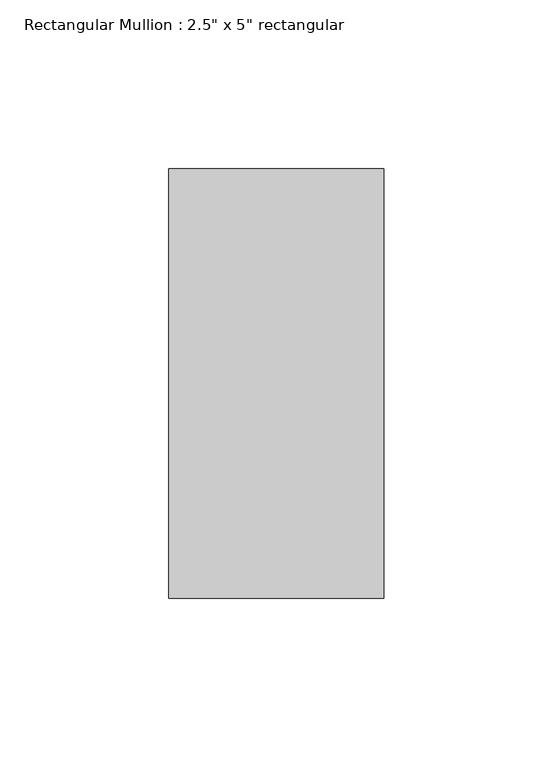
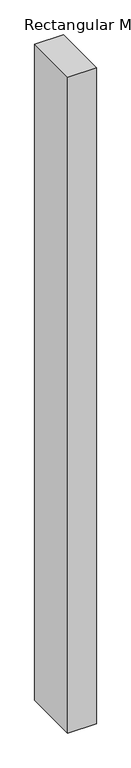
"""IFC4 building model written with IfcOpenShell, lengths in millimetres: member geometry."""

from ifc_helpers import new_model, si_unit, frame, origin, place, context, project, spatial, polyline, outline, extrude, source, transform, mapped, element, save


def member_957aaf5a(model_context):
    return source(origin(), model_context, "Body", "SweptSolid", [
        extrude(outline(polyline([(31.75, 63.5), (31.75, -63.5), (-31.75, -63.5), (-31.75, 63.5), (31.75, 63.5)])), frame((0.0, 0.0, -1539.437083), z_axis=(0.0, 0.0, 1.0), x_axis=(1.0, 0.0, 0.0)), (0.0, 0.0, 1.0), 1539.437083),
    ])


if __name__ == "__main__":
    model = new_model("IFC4")
    model_context = context("Model", 3, world=origin())
    ifc_project = project(units=[si_unit("LENGTHUNIT", "METRE", prefix="MILLI")], contexts=[model_context])
    site = spatial("IfcSite", under=ifc_project)
    building = spatial("IfcBuilding", under=site)
    placement = place(None, origin())
    member_shape = member_957aaf5a(model_context)
    element("IfcMember", 1, ObjectType="Rectangular Mullion : 2.5\" x 5\" rectangular", at=placement, inside=building, context=model_context, shape_type="MappedRepresentation", body=[
        mapped(member_shape, transform((0.0, 0.0, 0.0), x_axis=(1.0, 0.0, 0.0), y_axis=(0.0, 1.0, 0.0), z_axis=(0.0, 0.0, 1.0))),
    ])
    save(model, "model.ifc")

# Revit data of these elements
# Type "Rectangular Mullion : 2.5\" x 5\" rectangular"
#   built-in parameter 1007304 = 0.416667 (stored number, unit not read)
#   built-in parameter 1007301 = 0.104167 (stored number, unit not read)
#   built-in parameter 1007300 = 0.104167 (stored number, unit not read)
# Element 1 (IfcMember, "Rectangular Mullion : 2.5\" x 5\" rectangular")
#   Materials on its faces: "Aluminum"
# Materials
#   "Aluminum": class "Metal", colour RGB 247 247 247, transparency 0, Description = "Aluminum 6061", Cost = 0
